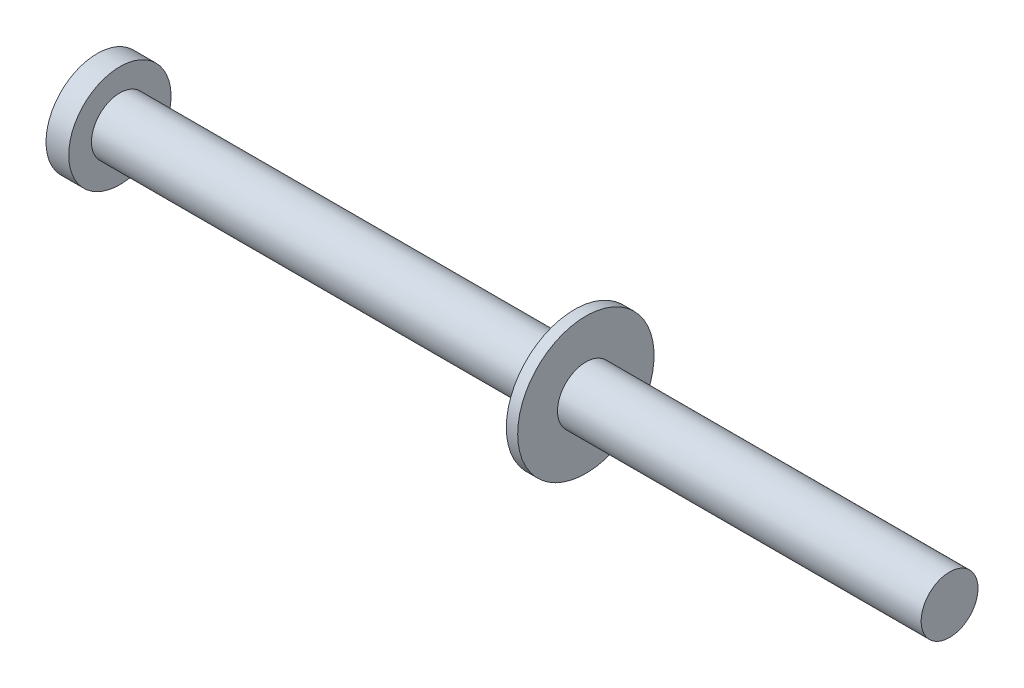
SolidWorks part; units mm, degrees
material "Plain Carbon Steel"
ref_plane "Front Plane" through (0, 0, 0) normal (0, 0, 1) x (1, 0, 0)
ref_plane "Top Plane" through (0, 0, 0) normal (0, 1, 0) x (1, 0, 0)
ref_plane "Right Plane" through (0, 0, 0) normal (1, 0, 0) x (0, 0, -1)
sketch "Shaft Section A Profile Ø10" plane through (0, 0, 0) normal (1, 0, 0) x (0, 0, -1)
  circle A0 centre (0, 0) radius 5
  dimension "D1" = 10
extrude "Shaft Section A Ø10x64" add sketch "Shaft Section A Profile Ø10" along normal blind 64
sketch "Collar Profile Ø24" plane through (0, 0, 0) normal (-1, 0, 0) x (0, 0, 1)
  circle A0 centre (0, 0) radius 12
  dimension "D1" = 24
extrude "Collar Ø24x2" add sketch "Collar Profile Ø24" along normal blind 2
sketch "Shaft Section B Profile Ø10" plane through (-2, 0, 0) normal (-1, 0, 0) x (0, 0, 1)
  circle A0 centre (0, 0) radius 5
  dimension "D1" = 10
extrude "Shaft Section B Ø10x80" add sketch "Shaft Section B Profile Ø10" along normal blind 80
sketch "Head Profile Ø18" plane through (-82, 0, 0) normal (-1, 0, 0) x (0, 0, 1)
  circle A0 centre (0, 0) radius 9
  dimension "D1" = 18
extrude "Head Ø18x4" add sketch "Head Profile Ø18" along normal blind 4
